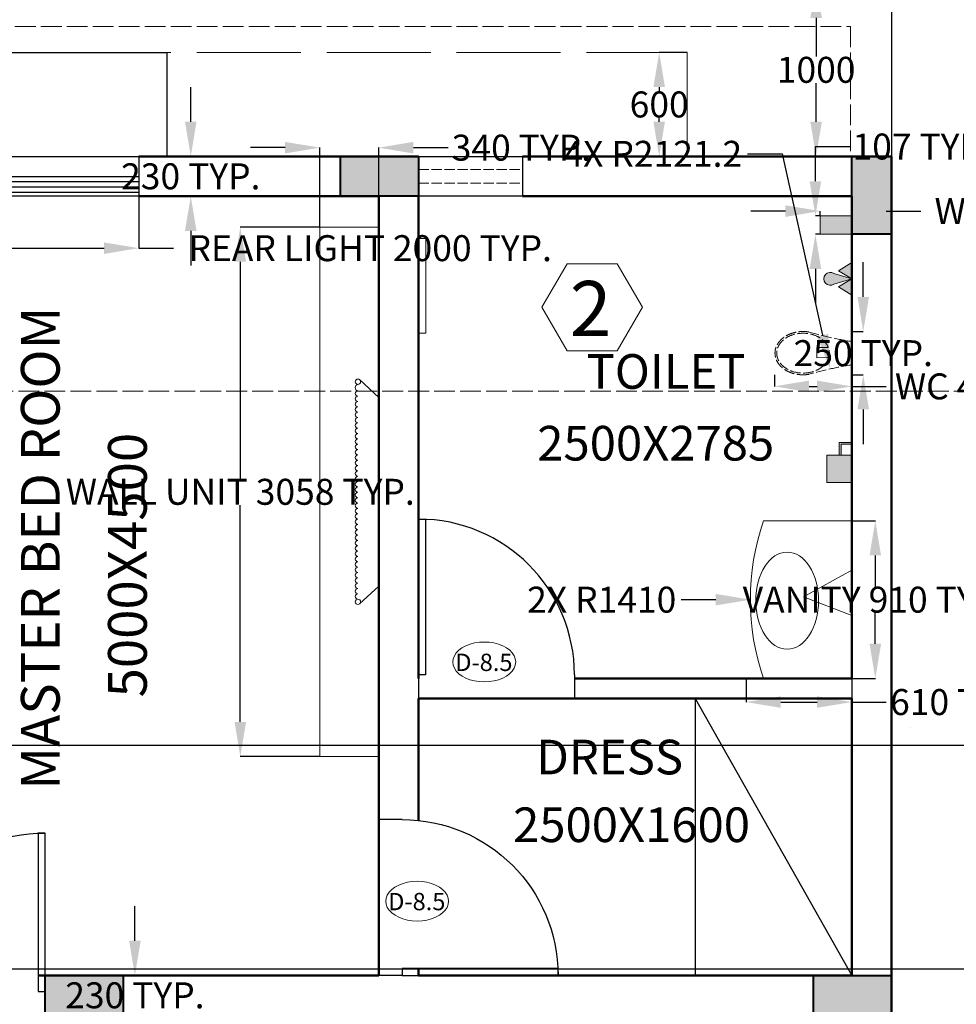
# Model space of a CAD drawing. Units: inches. Extents: x 22626 to 57351, y 2118 to 36234.
# Tile 8 of 10: x 44155 to 49561, y 23360 to 29046. Entities that reach past the tile are written whole.
import ezdxf

# ---------------------------------------------------------------- set-up
doc = ezdxf.new("R2010")
doc.units = ezdxf.units.IN
doc.header["$MEASUREMENT"] = 0
doc.linetypes.add('ACAD_ISO02W100', pattern=[15, 12, -3])
for name, color, linetype, lineweight in [('A-ANNO-DIMS', 130, 'Continuous', 18), ('A-ANNO-IDEN', 130, 'Continuous', 15), ('A-AREA-IDEN', 130, 'Continuous', 18), ('A-COLS', 7, 'Continuous', 40), ('A-COLS-PATT', 7, 'Continuous', 18), ('A-FLOR', 80, 'Continuous', 30), ('A-FLOR-CASE', 30, 'Continuous', 25), ('A-FLOR-FIXT', 30, 'Continuous', 18), ('A-FLOR-FIXT-HIDN', 30, 'ACAD_ISO02W100', 18), ('A-GLAZ-VENT', 152, 'Continuous', 25), ('A-GLAZ-VENT-HIDN', 152, 'ACAD_ISO02W100', 18), ('A-ROOF', 80, 'Continuous', 25), ('A-ROOF-OVHD', 80, 'ACAD_ISO02W100', 18), ('A-WALL', 80, 'Continuous', 50), ('DOORS', 32, 'Continuous', 25), ('FURNITURE', 30, 'Continuous', 18), ('WINDOWS', 212, 'Continuous', 25)]:
    doc.layers.add(name, color=color, linetype=linetype, lineweight=lineweight)
doc.layers.add('A-SECT', color=2, linetype='ACAD_ISO02W100', lineweight=18, true_color=0xf1eb1f)
doc.styles.get("Standard").update_dxf_attribs({"font": 'arial.ttf'})
doc.dimstyles.get("Standard").update_dxf_attribs({"dimtxt": 150, "dimasz": 200, "dimexe": 0.18, "dimexo": 0.0625, "dimgap": 0.09, "dimtad": 0, "dimtih": 1, "dimtoh": 1, "dimdec": 0, "dimzin": 0, "dimdsep": 46, "dimtxsty": 'Standard', "dimcen": 0.09, "dimadec": 0, "dimazin": 0, "dimtfac": 1, "dimtdec": 0, "dimtofl": 0, "dimtmove": 0, "dimatfit": 3, "dimfxl": 1, "dimtolj": 1, "dimtzin": 0, "dimarcsym": 0})

# ---------------------------------------------------------------- blocks, each defined once
blk = doc.blocks.new('*U7')
for p, q in [((0, 0), (-1e-16, -5.999999999999999)), ((40, -6e-16), (40, -6))]:
    blk.add_line(p, q)
blk.add_lwpolyline([(0, 0), (5.6e-15, 40), (1.750000000000007, 40), (1.749999999999998, -7e-16)], close=True)
blk.add_arc((0, 0), 40, 0, 90)
blk = doc.blocks.new('*D24')
at = {"layer": 'A-ANNO-DIMS', "color": 0, "lineweight": -2, "transparency": 16777216}
for p, q in [((48950.70212366983, 29256.86010836475), (48751.99162901918, 29256.86010836475)), ((48752.17162901917, 29056.86010836475), (48752.17162901917, 28833.536056523)), ((48752.17162901917, 28456.86010836475), (48752.17162901917, 28680.1841602065)), ((48950.70212366983, 28256.86010836474), (48751.99162901918, 28256.86010836474))]:
    blk.add_line(p, q, dxfattribs=at)
at = {"layer": 'A-ANNO-DIMS', "color": 0, "transparency": 16777216}
for points in [[(48718.83829568584, 29056.86010836475), (48785.50496235251, 29056.86010836475), (48752.17162901917, 29256.86010836475)], [(48718.83829568584, 28456.86010836475), (48785.50496235251, 28456.86010836475), (48752.17162901917, 28256.86010836474)]]:
    blk.add_solid(points, dxfattribs=at)
at = {"layer": 'Defpoints', "color": 0, "transparency": 16777216}
for p in [(48752.17162901917, 29256.86010836475), (48950.76462366983, 29256.86010836475), (48950.76462366983, 28256.86010836474)]:
    blk.add_point(p, dxfattribs=at)
at = {"layer": 'A-ANNO-DIMS', "color": 0, "transparency": 16777216, "insert": (48752.17162901917, 28756.86010836473), "char_height": 150, "attachment_point": 5}
blk.add_mtext('\\A1;1000', dxfattribs=at)
blk = doc.blocks.new('*D25')
at = {"layer": 'A-ANNO-DIMS', "color": 0, "lineweight": -2, "transparency": 16777216}
for p, q in [((48007.78103641213, 28856.86010836474), (47846.08778381056, 28856.86010836474)), ((47846.26778381056, 28656.86010836475), (47846.26778381056, 28633.536056523)), ((47846.26778381056, 28456.86010836475), (47846.26778381056, 28480.18416020649)), ((48007.78103641213, 28256.86010836474), (47846.08778381056, 28256.86010836474))]:
    blk.add_line(p, q, dxfattribs=at)
at = {"layer": 'A-ANNO-DIMS', "color": 0, "transparency": 16777216}
for points in [[(47812.93445047722, 28656.86010836475), (47879.6011171439, 28656.86010836475), (47846.26778381056, 28856.86010836474)], [(47812.93445047722, 28456.86010836475), (47879.6011171439, 28456.86010836475), (47846.26778381056, 28256.86010836474)]]:
    blk.add_solid(points, dxfattribs=at)
at = {"layer": 'Defpoints', "color": 0, "transparency": 16777216}
for p in [(47846.26778381056, 28856.86010836474), (48007.84353641212, 28856.86010836474), (48007.84353641212, 28256.86010836474)]:
    blk.add_point(p, dxfattribs=at)
at = {"layer": 'A-ANNO-DIMS', "color": 0, "transparency": 16777216, "insert": (47846.26778381056, 28556.86010836473), "char_height": 150, "attachment_point": 5}
blk.add_mtext('\\A1;600', dxfattribs=at)
blk = doc.blocks.new('BEDROOM-WALL-UNIT-LARGE')
for p, q in [((340.3900439586505, 2073.364799085331), (230.0040754163856, 2176.56373781851)), ((340.3900439586505, 2073.364799085331), (340.3900439586505, 984.3248137472802)), ((340.3900439586505, 984.3248137472802), (230.0040754163856, 881.1258750141023))]:
    blk.add_line(p, q)
blk.add_lwpolyline([(340.3900439586505, 3057.689448538677), (0.000138100287586, 3057.689448538677), (0.000138100287586, 0.0001642939350859), (340.3900439586505, 0.0001642939350859)], close=True)
for centre in [(220.3862887798459, 2164.500040820422), (220.3862887798459, 893.1895720121902)]:
    blk.add_circle(centre, 15.42837013581516)
for centre, radius, start, end in [((223.4783476155644, 2130.551241713074), 18.77677067903697, 99.47833690620159, 260.5216630937984), ((220.3862887798459, 2096.602442605719), 15.42837013581516, 90, 270), ((220.3862887798459, 2065.745702334091), 15.42837013581516, 90, 270), ((220.3862887798459, 2034.888962062462), 15.42837013581516, 90, 270), ((220.3862887798459, 2004.032221790833), 15.42837013581516, 90, 270), ((220.3862887798459, 1973.175481519203), 15.42837013581516, 90, 270), ((220.3862887798459, 1942.318741247574), 15.42837013581516, 90, 270), ((220.3862887798459, 1911.462000975945), 15.42837013581516, 90, 270), ((220.3862887798459, 1880.605260704317), 15.42837013581516, 90, 270), ((220.3862887798459, 1849.748520432688), 15.42837013581516, 90, 270), ((220.3862887798459, 1818.891780161058), 15.42837013581516, 90, 270), ((220.3862887798459, 1788.03503988943), 15.42837013581516, 90, 270), ((220.3862887798459, 1757.178299617801), 15.42837013581516, 90, 270), ((220.3862887798459, 1726.321559346172), 15.42837013581516, 90, 270), ((220.3862887798459, 1695.464819074543), 15.42837013581516, 90, 270), ((220.3862887798459, 1664.608078802914), 15.42837013581516, 90, 270), ((220.3862887798459, 1633.751338531285), 15.42837013581516, 90, 270), ((220.3862887798459, 1602.894598259656), 15.42837013581516, 90, 270), ((220.3862887798459, 1572.037857988027), 15.42837013581516, 90, 270), ((220.3862887798459, 1541.181117716398), 15.42837013581516, 90, 270), ((220.3862887798459, 1510.324377444769), 15.42837013581516, 90, 270), ((220.3862887798459, 1479.46763717314), 15.42837013581516, 90, 270), ((220.3862887798459, 1448.610896901511), 15.42837013581516, 90, 270), ((220.3862887798459, 1417.754156629882), 15.42837013581516, 90, 270), ((220.3862887798459, 1386.897416358253), 15.42837013581516, 90, 270), ((220.3862887798459, 1356.040676086624), 15.42837013581516, 90, 270), ((220.3862887798459, 1325.183935814995), 15.42837013581516, 90, 270), ((220.3862887798459, 1294.327195543366), 15.42837013581516, 90, 270), ((220.3862887798459, 1263.470455271737), 15.42837013581516, 90, 270), ((220.3862887798459, 1232.613715000108), 15.42837013581516, 90, 270), ((220.3862887798459, 1201.756974728479), 15.42837013581516, 90, 270), ((220.3862887798459, 1170.90023445685), 15.42837013581516, 90, 270), ((220.3862887798459, 1140.043494185221), 15.42837013581516, 90, 270), ((220.3862887798459, 1109.186753913593), 15.42837013581516, 90, 270), ((220.3862887798459, 1078.330013641964), 15.42837013581516, 90, 270), ((220.3862887798459, 1047.473273370335), 15.42837013581516, 90, 270), ((220.3862887798459, 1016.616533098706), 15.42837013581516, 90, 270), ((220.3862887798459, 985.759792827077), 15.42837013581516, 90, 270), ((220.3862887798459, 954.9030525554481), 15.42837013581516, 90, 270), ((220.3862887798459, 924.0463122838191), 15.42837013581516, 90, 270)]:
    blk.add_arc(centre, radius, start, end)
blk = doc.blocks.new('WC')
at = {"ltscale": 5}
for p, q in [((307.4540408789253, 157.9229967620813), (242.2174300020561, 157.9229967620813)), ((242.2174300020561, 157.9229967620813), (242.2174300020561, 97.87988847275483)), ((307.4540408789253, 157.9229967620813), (307.4540408789253, 157.9229967620813)), ((242.2174300020561, 97.87988847275483), (310.0842174796853, 99.70460823710528))]:
    blk.add_line(p, q, dxfattribs=at)
for centre, start, end in [((780.732508801062, 2286.288249576111), 254.000576969056, 260.8285458946419), ((780.732508801062, -2036.267674000785), 99.17145410535805, 105.999423030944)]:
    blk.add_arc(centre, 2121.236142909723, start, end, dxfattribs=at)
blk.add_ellipse((161.9027973060947, 125.0102877876634), major_axis=(151.9040759523413, 0), ratio=0.7571275708385353, start_param=-1.570796326794896, end_param=4.712388980384689, dxfattribs=at)
for points, knots in [([(196.0611207178517, 247.2193096078299), (189.9898489161132, 248.2266596507652), (183.8456655129121, 248.9650412442752), (168.6182293347155, 250.1102459839712), (159.4964975931143, 250.2034131541222), (141.3581357193834, 249.212698022955), (132.3417047420516, 248.1288311957833), (114.6613914742556, 244.8098406800164), (105.9976853845146, 242.5747636017513), (89.26201623554518, 237.0062334978611), (81.19018288652298, 233.6728365616509), (65.86452451616788, 225.9859897466813), (58.61077128878969, 221.6325587335632), (45.13156838521536, 212.0080719868456), (38.90616664764093, 206.7369257869286), (27.67640637096338, 195.4043234284545), (22.67220516936504, 189.3426231032536), (14.05759261523781, 176.5860631599644), (10.44766267286468, 169.8909471035294), (4.765577569938614, 156.0629077761186), (2.69424158098991, 148.9301527436837), (0.1846293913040426, 134.463597005164), (-0.2530317139462568, 127.1307025187488), (0.5271766823570943, 112.5265070110981), (1.744832412616233, 105.2563518462193), (5.77749157987273, 91.03263116568269), (8.591685077881264, 84.07962673572185), (15.69573821845551, 70.70922901844096), (19.98490811580268, 64.29173781119243), (29.87879523489392, 52.16900764399179), (35.483208879421, 46.46348057011346), (47.82439502190391, 35.90657261581146), (54.56108629030495, 31.05501885116246), (68.96556532807881, 22.32099587028279), (76.63330319123634, 18.43849746629348), (92.68186228567357, 11.73355477496807), (101.0625846676266, 8.91115468616772), (118.3043576900527, 4.392898517646244), (127.1652540279829, 2.697098106120392), (144.6597339432555, 0.5298149587142689), (153.2812269904534, -0.000476238605188), (161.9027973060947, -0.000476238605188)], [1.35503494441986, 1.35503494441986, 1.35503494441986, 1.35503494441986, 1.471789532681877, 1.471789532681877, 1.642812487519809, 1.642812487519809, 1.813835442357741, 1.813835442357741, 1.984858397195673, 1.984858397195673, 2.155881352033606, 2.155881352033606, 2.326904306871538, 2.326904306871538, 2.49792726170947, 2.49792726170947, 2.668950216547402, 2.668950216547402, 2.839973171385334, 2.839973171385334, 3.010996126223266, 3.010996126223266, 3.182019081061198, 3.182019081061198, 3.35304203589913, 3.35304203589913, 3.524064990737062, 3.524064990737062, 3.695087945574994, 3.695087945574994, 3.866110900412926, 3.866110900412926, 4.037133855250859, 4.037133855250859, 4.208156810088791, 4.208156810088791, 4.379179764926723, 4.379179764926723, 4.550202719764655, 4.550202719764655, 4.712388980384689, 4.712388980384689, 4.712388980384689, 4.712388980384689]), ([(161.9027973060947, -0.000476238605188), (167.8851873344465, -0.000476238605188), (173.8675648995122, 0.254611844480678), (185.2699231324077, 1.230286525809788), (190.6953945214336, 1.911114408936555), (196.0639028232108, 2.802063691000512)], [-1.570796326794896, -1.570796326794896, -1.570796326794896, -1.570796326794896, -1.458257493061962, -1.458257493061962, -1.355016516099114, -1.355016516099114, -1.355016516099114, -1.355016516099114])]:
    blk.add_open_spline(points, degree=3, knots=knots, dxfattribs=at)
blk = doc.blocks.new('VANITY-BASIN')
for p, q in [((584.7220439586453, 910.0402479339828), (75.43762569876708, 910.0402479339828)), ((305.8230790732414, 471.9850997598696), (584.7220439586453, 624.7406586797733)), ((305.8230790732414, 471.9850997598696), (584.7220439586453, 362.8739423048537))]:
    blk.add_line(p, q)
blk.add_arc((1409.991080111897, 455.0201781493488), 1409.991555504085, 161.1730336158717, 198.8269663841282)
blk.add_ellipse((212.5566461408889, 449.1359101998277), major_axis=(0, -280.3059750137254), ratio=0.6469075979310198)
blk = doc.blocks.new('WIN-FIXED-2000-REAR')
for p, q in [((4.39586510765e-05, 114.2630103577103), (2000.000043958651, 114.2630103577103)), ((4.39586510765e-05, 84.26301035771031), (2000.000043958651, 84.26301035771031)), ((4.39586510765e-05, 54.2630103577103), (2000.000043958651, 54.2630103577103)), ((4.39586510765e-05, 24.2630103577103), (2000.000043958651, 24.2630103577103))]:
    blk.add_line(p, q)
blk.add_lwpolyline([(4.39586510765e-05, 230.0001083647294), (2000.000043958651, 230.0001083647294), (2000.000043958651, 0.0001083647330233), (4.39586438006e-05, 0.0001083647330233), (4.39586510765e-05, 230.0001083647294)])
blk = doc.blocks.new('COL-RECTANGULAR')
h = blk.add_hatch(color=256)
h.dxf.hatch_style = 1
h.paths.add_polyline_path([(4.39586474386e-05, 0.0001083647293854), (450.0000439586474, 0.0001083647293854), (450.0000439586474, 230.0001083647294), (4.39586474386e-05, 230.0001083647294)])
blk.add_lwpolyline([(4.39586474386e-05, 0.0001083647293854), (4.39586474386e-05, 230.0001083647294), (450.0000439586474, 230.0001083647294), (450.0000439586474, 0.0001083647293854)], close=True)
blk = doc.blocks.new('BATH-SUPPLY-FITTING')
h = blk.add_hatch(color=256)
h.dxf.hatch_style = 1
h.paths.add_polyline_path([(161.0140439586466, 189.3806798614205), (84.84003036547074, 140.983449503361), (161.0140439586466, 94.69046873241678)])
h = blk.add_hatch(color=256)
h.dxf.hatch_style = 1
h.paths.add_polyline_path([(161.0140439586466, 94.69046873241678), (58.24591656582924, 125.2086534748123, 1.90856376211952), (58.24591656582924, 64.17228399002124)])
h = blk.add_hatch(color=256)
h.dxf.hatch_style = 1
h.paths.add_polyline_path([(161.0140439586466, 94.69046873241678), (84.84003036547074, 48.39748796147251), (161.0140439586466, 0.000257603413047)])
for p, q in [((161.0140439586466, 189.3806798614205), (84.84003036547074, 140.983449503361)), ((161.0140439586466, 94.69046873241678), (58.24591656582924, 125.2086534748123)), ((84.84003036547074, 140.983449503361), (161.0140439586466, 94.69046873241678)), ((161.0140439586466, 94.69046873241678), (58.24591656582924, 64.17228399002124)), ((84.84003036547074, 48.39748796147251), (161.0140439586466, 94.69046873241678)), ((161.0140439586466, 0.000257603413047), (84.84003036547074, 48.39748796147251))]:
    blk.add_line(p, q)
blk.add_arc((37.11803136635718, 94.69046873241678), 37.11801628553248, 55.30495923588778, 304.6950407641123)
blk = doc.blocks.new('BATH-WALL-ACCESSORY')
h = blk.add_hatch(color=256)
h.dxf.hatch_style = 1
h.paths.add_polyline_path([(142.8430439586445, 231.1050653827879), (71.42162994010141, 231.1050653827879), (71.42162994010141, 158.5160872540764), (81.4216299401014, 158.5160872540764), (81.42162994010869, 221.1050653827879), (142.8430439586445, 221.1050653827879)])
h = blk.add_hatch(color=256)
h.dxf.hatch_style = 1
h.paths.add_polyline_path([(142.8430439586445, 158.5160872540764), (0.0002159215582651, 158.5160872540764), (0.0002159215582651, -1.22242890939e-05), (142.8430439586445, -1.22242854559e-05)])
for p, q in [((71.42162994010141, 158.5160872540764), (71.42162994010141, 231.1050653827879)), ((71.42162994010141, 231.1050653827879), (142.8430439586445, 231.1050653827879)), ((81.42162994010869, 221.1050653827879), (142.8430439586445, 221.1050653827879)), ((81.4216299401014, 158.5160872540764), (81.42162994010869, 221.1050653827879)), ((142.8430439586445, 158.5160872540764), (0.0002159215582651, 158.5160872540764)), ((0.0002159215582651, 158.5160872540764), (0.0002159215582651, -1.22242890939e-05)), ((142.8430439586445, 158.5160872540764), (142.8430439586445, 158.5160872540764)), ((0.0002159215582651, -1.22242890939e-05), (142.8430439586445, -1.22242854559e-05))]:
    blk.add_line(p, q)
blk = doc.blocks.new('BATH-WALL-BOX')
h = blk.add_hatch(color=256)
h.dxf.hatch_style = 1
h.paths.add_polyline_path([(182.0210439586444, 106.8341357510071), (0.000183795193152, 106.8341357510071), (0.000183795193152, 0.0001083647293854), (182.0210439586444, 0.0001083647293854)])
for p, q in [((0.000183795193152, 0.0001083647293854), (0.000183795193152, 106.8341357510071)), ((0.000183795193152, 106.8341357510071), (182.0210439586444, 106.8341357510071)), ((182.0210439586444, 0.0001083647293854), (0.000183795193152, 0.0001083647293854))]:
    blk.add_line(p, q)
blk = doc.blocks.new('WINDOW-HOOD')
for p, q in [((-0.0002120264252881, 0.0001083647293854), (-0.0002120264252881, 600.0001083647293)), ((-0.0002120264252881, 600.0001083647293), (2314.590014351226, 600.0001083647293)), ((2314.590014351226, 600.0001083647293), (2314.590014351226, 0.0001083647330233))]:
    blk.add_line(p, q)
blk = doc.blocks.new('*D56')
at = {"layer": 'A-ANNO-DIMS', "color": 0, "lineweight": -2, "transparency": 16777216}
for p, q in [((44302.42904395863, 23296.79760836473), (44302.42904395863, 23229.18010836473)), ((44752.42904395862, 23296.79760836473), (44752.42904395862, 23229.18010836473)), ((44502.42904395863, 23229.36010836473), (44552.42904395862, 23229.36010836473)), ((44752.42904395862, 23229.36010836473), (44952.42904395862, 23229.36010836473))]:
    blk.add_line(p, q, dxfattribs=at)
at = {"layer": 'A-ANNO-DIMS', "color": 0, "transparency": 16777216}
for points in [[(44502.42904395863, 23262.69344169806), (44502.42904395863, 23196.0267750314), (44302.42904395863, 23229.36010836473)], [(44552.42904395862, 23262.69344169806), (44552.42904395862, 23196.0267750314), (44752.42904395862, 23229.36010836473)]]:
    blk.add_solid(points, dxfattribs=at)
at = {"layer": 'Defpoints', "color": 0, "transparency": 16777216}
for p in [(44302.42904395863, 23296.86010836473), (44752.42904395862, 23296.86010836473), (44752.42904395862, 23229.36010836473)]:
    blk.add_point(p, dxfattribs=at)
at = {"layer": 'A-ANNO-DIMS', "color": 0, "transparency": 16777216, "insert": (45858.14660193952, 23229.36010836473), "char_height": 150, "attachment_point": 5}
blk.add_mtext('\\A1;COLUMN 450 TYP.', dxfattribs=at)
blk = doc.blocks.new('*D57')
at = {"layer": 'A-ANNO-DIMS', "color": 0, "lineweight": -2, "transparency": 16777216}
for p, q in [((44819.92904395865, 23726.86010836474), (44819.92904395865, 23926.86010836474)), ((44752.49154395863, 23526.86010836474), (44820.10904395865, 23526.86010836474)), ((44752.49154395863, 23296.86010836474), (44820.10904395865, 23296.86010836474)), ((44819.92904395865, 23096.86010836474), (44819.92904395865, 22896.86010836474))]:
    blk.add_line(p, q, dxfattribs=at)
at = {"layer": 'A-ANNO-DIMS', "color": 0, "transparency": 16777216}
for points in [[(44786.59571062531, 23726.86010836474), (44853.26237729199, 23726.86010836474), (44819.92904395865, 23526.86010836474)], [(44786.59571062531, 23096.86010836474), (44853.26237729199, 23096.86010836474), (44819.92904395865, 23296.86010836474)]]:
    blk.add_solid(points, dxfattribs=at)
at = {"layer": 'Defpoints', "color": 0, "transparency": 16777216}
for p in [(44752.42904395864, 23526.86010836474), (44819.92904395865, 23526.86010836474), (44752.42904395864, 23296.86010836474)]:
    blk.add_point(p, dxfattribs=at)
at = {"layer": 'A-ANNO-DIMS', "color": 0, "transparency": 16777216, "insert": (44819.92904395865, 23411.86010836472), "char_height": 150, "attachment_point": 5}
blk.add_mtext('\\A1;230 TYP.', dxfattribs=at)
blk = doc.blocks.new('*D62')
at = {"layer": 'A-ANNO-DIMS', "color": 0, "lineweight": -2, "transparency": 16777216}
for p, q in [((48511.89638763924, 26995.3910237614), (48511.89638763924, 26928.44362531275)), ((48957.42904396353, 26995.3910237614), (48957.42904396353, 26928.44362531275)), ((48711.89638763923, 26928.62362531275), (48757.42904396354, 26928.62362531275)), ((48957.42904396353, 26928.62362531275), (49157.42904396354, 26928.62362531275))]:
    blk.add_line(p, q, dxfattribs=at)
at = {"layer": 'A-ANNO-DIMS', "color": 0, "transparency": 16777216}
for points in [[(48711.89638763923, 26961.95695864608), (48711.89638763923, 26895.29029197942), (48511.89638763924, 26928.62362531275)], [(48757.42904396354, 26961.95695864608), (48757.42904396354, 26895.29029197942), (48957.42904396353, 26928.62362531275)]]:
    blk.add_solid(points, dxfattribs=at)
at = {"layer": 'Defpoints', "color": 0, "transparency": 16777216}
for p in [(48511.89638763924, 26995.4535237614), (48957.42904396353, 26995.4535237614), (48957.42904396353, 26928.62362531275)]:
    blk.add_point(p, dxfattribs=at)
at = {"layer": 'A-ANNO-DIMS', "color": 0, "transparency": 16777216, "insert": (49787.60089935235, 26928.62362531275), "char_height": 150, "attachment_point": 5}
blk.add_mtext('\\A1;WC 446 TYP.', dxfattribs=at)
blk = doc.blocks.new('*D63')
at = {"layer": 'A-ANNO-DIMS', "color": 0, "lineweight": -2, "transparency": 16777216}
for p, q in [((49024.25894241221, 27445.65741315414), (49024.25894241221, 27645.65741315414)), ((48957.49154396355, 27245.65741315414), (49024.43894241221, 27245.65741315414)), ((48957.49154396355, 26995.45352376141), (49024.43894241221, 26995.45352376141)), ((49024.25894241221, 26795.45352376141), (49024.25894241221, 26595.45352376141))]:
    blk.add_line(p, q, dxfattribs=at)
at = {"layer": 'A-ANNO-DIMS', "color": 0, "transparency": 16777216}
for points in [[(48990.92560907887, 27445.65741315414), (49057.59227574555, 27445.65741315414), (49024.25894241221, 27245.65741315414)], [(48990.92560907887, 26795.45352376141), (49057.59227574555, 26795.45352376141), (49024.25894241221, 26995.45352376141)]]:
    blk.add_solid(points, dxfattribs=at)
at = {"layer": 'Defpoints', "color": 0, "transparency": 16777216}
for p in [(48957.42904396355, 27245.65741315414), (49024.25894241221, 27245.65741315414), (48957.42904396355, 26995.45352376141)]:
    blk.add_point(p, dxfattribs=at)
at = {"layer": 'A-ANNO-DIMS', "color": 0, "transparency": 16777216, "insert": (49024.25894241221, 27120.55546845776), "char_height": 150, "attachment_point": 5}
blk.add_mtext('\\A1;250 TYP.', dxfattribs=at)
blk = doc.blocks.new('*D64')
at = {"layer": 'A-ANNO-DIMS', "color": 0, "lineweight": -2, "transparency": 16777216}
for p, q in [((48957.49154395866, 26151.900247934), (49094.1150648939, 26151.900247934)), ((49093.9350648939, 25951.900247934), (49093.9350648939, 25773.55612630816)), ((49093.9350648939, 25441.86010836582), (49093.9350648939, 25620.20422999166)), ((48957.49154395866, 25241.86010836582), (49094.1150648939, 25241.86010836582))]:
    blk.add_line(p, q, dxfattribs=at)
at = {"layer": 'A-ANNO-DIMS', "color": 0, "transparency": 16777216}
for points in [[(49060.60173156056, 25951.900247934), (49127.26839822723, 25951.900247934), (49093.9350648939, 26151.900247934)], [(49060.60173156056, 25441.86010836582), (49127.26839822723, 25441.86010836582), (49093.9350648939, 25241.86010836582)]]:
    blk.add_solid(points, dxfattribs=at)
at = {"layer": 'Defpoints', "color": 0, "transparency": 16777216}
for p in [(48957.42904395866, 26151.900247934), (49093.9350648939, 26151.900247934), (48957.42904395866, 25241.86010836582)]:
    blk.add_point(p, dxfattribs=at)
at = {"layer": 'A-ANNO-DIMS', "color": 0, "transparency": 16777216, "insert": (49093.9350648939, 25696.88017814989), "char_height": 150, "attachment_point": 5}
blk.add_mtext('\\A1;VANITY 910 TYP.', dxfattribs=at)
blk = doc.blocks.new('*D65')
at = {"layer": 'A-ANNO-DIMS', "color": 0, "lineweight": -2, "transparency": 16777216}
for p, q in [((48347.56049091095, 25241.79760836581), (48347.56049091095, 25105.17408743058)), ((48957.42904395865, 25241.79760836581), (48957.42904395865, 25105.17408743058)), ((48547.56049091095, 25105.35408743058), (48757.42904395864, 25105.35408743058)), ((48957.42904395865, 25105.35408743058), (49157.42904395864, 25105.35408743058))]:
    blk.add_line(p, q, dxfattribs=at)
at = {"layer": 'A-ANNO-DIMS', "color": 0, "transparency": 16777216}
for points in [[(48547.56049091095, 25138.68742076391), (48547.56049091095, 25072.02075409725), (48347.56049091095, 25105.35408743058)], [(48757.42904395864, 25138.68742076391), (48757.42904395864, 25072.02075409725), (48957.42904395865, 25105.35408743058)]]:
    blk.add_solid(points, dxfattribs=at)
at = {"layer": 'Defpoints', "color": 0, "transparency": 16777216}
for p in [(48347.56049091095, 25241.86010836581), (48957.42904395865, 25241.86010836581), (48957.42904395865, 25105.35408743058)]:
    blk.add_point(p, dxfattribs=at)
at = {"layer": 'A-ANNO-DIMS', "color": 0, "transparency": 16777216, "insert": (49581.27415992044, 25105.35408743058), "char_height": 150, "attachment_point": 5}
blk.add_mtext('\\A1;610 TYP.', dxfattribs=at)
blk = doc.blocks.new('*D70')
at = {"layer": 'A-ANNO-DIMS', "color": 0, "lineweight": -2, "transparency": 16777216}
for p, q in [((48575.4081837952, 27940.99726477552), (48375.4081837952, 27940.99726477552)), ((48775.4081837952, 27913.75663575101), (48775.4081837952, 27941.17726477553)), ((48957.42904395865, 27913.75663575101), (48957.42904395865, 27941.17726477553)), ((49157.42904395864, 27940.99726477552), (49357.42904395865, 27940.99726477552))]:
    blk.add_line(p, q, dxfattribs=at)
at = {"layer": 'A-ANNO-DIMS', "color": 0, "transparency": 16777216}
for points in [[(48575.4081837952, 27974.33059810886), (48575.4081837952, 27907.66393144219), (48775.4081837952, 27940.99726477552)], [(49157.42904395864, 27974.33059810886), (49157.42904395864, 27907.66393144219), (48957.42904395865, 27940.99726477552)]]:
    blk.add_solid(points, dxfattribs=at)
at = {"layer": 'Defpoints', "color": 0, "transparency": 16777216}
for p in [(48957.42904395865, 27940.99726477552), (48775.4081837952, 27913.69413575101), (48957.42904395865, 27913.69413575101)]:
    blk.add_point(p, dxfattribs=at)
at = {"layer": 'A-ANNO-DIMS', "color": 0, "transparency": 16777216, "insert": (50348.73664286724, 27940.99726477552), "char_height": 150, "attachment_point": 5}
blk.add_mtext('\\A1;WALL BOX 182 TYP.', dxfattribs=at)
blk = doc.blocks.new('*D71')
at = {"layer": 'A-ANNO-DIMS', "color": 0, "lineweight": -2, "transparency": 16777216}
for p, q in [((48748.1050547707, 28113.69413575102), (48748.1050547707, 28313.69413575102)), ((48748.1050547707, 28313.69413575102), (48948.10505477069, 28313.69413575102)), ((48775.34568379521, 27913.69413575102), (48747.9250547707, 27913.69413575102)), ((48775.34568379521, 27806.86010836475), (48747.9250547707, 27806.86010836475)), ((48748.1050547707, 27606.86010836475), (48748.1050547707, 27406.86010836475))]:
    blk.add_line(p, q, dxfattribs=at)
at = {"layer": 'A-ANNO-DIMS', "color": 0, "transparency": 16777216}
for points in [[(48714.77172143736, 28113.69413575102), (48781.43838810403, 28113.69413575102), (48748.1050547707, 27913.69413575102)], [(48714.77172143736, 27606.86010836475), (48781.43838810403, 27606.86010836475), (48748.1050547707, 27806.86010836475)]]:
    blk.add_solid(points, dxfattribs=at)
at = {"layer": 'Defpoints', "color": 0, "transparency": 16777216}
for p in [(48748.1050547707, 27913.69413575102), (48775.40818379522, 27913.69413575102), (48775.40818379522, 27806.86010836475)]:
    blk.add_point(p, dxfattribs=at)
at = {"layer": 'A-ANNO-DIMS', "color": 0, "transparency": 16777216, "insert": (49364.4808665033, 28313.694135751), "char_height": 150, "attachment_point": 5}
blk.add_mtext('\\A1;107 TYP.', dxfattribs=at)
blk = doc.blocks.new('*D78')
at = {"layer": 'A-ANNO-DIMS', "color": 0, "lineweight": -2, "transparency": 16777216}
for p, q in [((45886.97663810028, 27848.6944485387), (45428.20574546359, 27848.6944485387)), ((45428.38574546359, 27648.6944485387), (45428.38574546359, 26396.57691419259)), ((45428.38574546359, 24991.00516429395), (45428.38574546359, 26243.12269864006)), ((45886.97663810028, 24791.00516429395), (45428.20574546359, 24791.00516429395))]:
    blk.add_line(p, q, dxfattribs=at)
at = {"layer": 'A-ANNO-DIMS', "color": 0, "transparency": 16777216}
for points in [[(45395.05241213025, 27648.6944485387), (45461.71907879693, 27648.6944485387), (45428.38574546359, 27848.6944485387)], [(45395.05241213025, 24991.00516429395), (45461.71907879693, 24991.00516429395), (45428.38574546359, 24791.00516429395)]]:
    blk.add_solid(points, dxfattribs=at)
at = {"layer": 'Defpoints', "color": 0, "transparency": 16777216}
for p in [(45428.38574546359, 27848.6944485387), (45887.03913810029, 27848.6944485387), (45887.03913810029, 24791.00516429395)]:
    blk.add_point(p, dxfattribs=at)
at = {"layer": 'A-ANNO-DIMS', "color": 0, "transparency": 16777216, "insert": (45428.38574546359, 26319.8498064163), "char_height": 150, "attachment_point": 5}
blk.add_mtext('\\A1;WALL UNIT 3058 TYP.', dxfattribs=at)
blk = doc.blocks.new('*D79')
at = {"layer": 'A-ANNO-DIMS', "color": 0, "lineweight": -2, "transparency": 16777216}
for p, q in [((45687.03913810027, 28307.34784117539), (45487.03913810028, 28307.34784117539)), ((45887.03913810028, 27848.75694853868), (45887.03913810028, 28307.52784117539)), ((46227.42904395864, 27848.75694853868), (46227.42904395864, 28307.52784117539)), ((46427.42904395864, 28307.34784117539), (46627.42904395864, 28307.34784117539))]:
    blk.add_line(p, q, dxfattribs=at)
at = {"layer": 'A-ANNO-DIMS', "color": 0, "transparency": 16777216}
for points in [[(45687.03913810027, 28340.68117450872), (45687.03913810027, 28274.01450784206), (45887.03913810028, 28307.34784117539)], [(46427.42904395864, 28340.68117450872), (46427.42904395864, 28274.01450784206), (46227.42904395864, 28307.34784117539)]]:
    blk.add_solid(points, dxfattribs=at)
at = {"layer": 'Defpoints', "color": 0, "transparency": 16777216}
for p in [(46227.42904395864, 28307.34784117539), (45887.03913810028, 27848.69444853868), (46227.42904395864, 27848.69444853868)]:
    blk.add_point(p, dxfattribs=at)
at = {"layer": 'A-ANNO-DIMS', "color": 0, "transparency": 16777216, "insert": (47050.81372335837, 28307.34784117539), "char_height": 150, "attachment_point": 5}
blk.add_mtext('\\A1;340 TYP.', dxfattribs=at)
blk = doc.blocks.new('*D82')
at = {"layer": 'A-ANNO-DIMS', "color": 0, "lineweight": -2, "transparency": 16777216}
for p, q in [((42842.42904395863, 28026.79760836474), (42842.42904395863, 27726.68010836474)), ((44842.42904395864, 28026.79760836474), (44842.42904395864, 27726.68010836474)), ((43042.42904395863, 27726.86010836474), (44642.42904395864, 27726.86010836474)), ((44842.42904395864, 27726.86010836474), (45042.42904395864, 27726.86010836474))]:
    blk.add_line(p, q, dxfattribs=at)
at = {"layer": 'A-ANNO-DIMS', "color": 0, "transparency": 16777216}
for points in [[(43042.42904395863, 27760.19344169807), (43042.42904395863, 27693.52677503141), (42842.42904395863, 27726.86010836474)], [(44642.42904395864, 27760.19344169807), (44642.42904395864, 27693.52677503141), (44842.42904395864, 27726.86010836474)]]:
    blk.add_solid(points, dxfattribs=at)
at = {"layer": 'Defpoints', "color": 0, "transparency": 16777216}
for p in [(42842.42904395863, 28026.86010836474), (44842.42904395864, 28026.86010836474), (44842.42904395864, 27726.86010836474)]:
    blk.add_point(p, dxfattribs=at)
at = {"layer": 'A-ANNO-DIMS', "color": 0, "transparency": 16777216, "insert": (46178.10908488633, 27726.86010836474), "char_height": 150, "attachment_point": 5}
blk.add_mtext('\\A1;REAR LIGHT 2000 TYP.', dxfattribs=at)
blk = doc.blocks.new('*D83')
at = {"layer": 'A-ANNO-DIMS', "color": 0, "lineweight": -2, "transparency": 16777216}
for p, q in [((45142.42904395866, 28456.86010836475), (45142.42904395866, 28656.86010836475)), ((44842.49154395866, 28256.86010836474), (45142.60904395866, 28256.86010836474)), ((44842.49154395866, 28026.86010836475), (45142.60904395866, 28026.86010836475)), ((45142.42904395866, 27826.86010836475), (45142.42904395866, 27626.86010836475))]:
    blk.add_line(p, q, dxfattribs=at)
at = {"layer": 'A-ANNO-DIMS', "color": 0, "transparency": 16777216}
for points in [[(45109.09571062533, 28456.86010836475), (45175.762377292, 28456.86010836475), (45142.42904395866, 28256.86010836474)], [(45109.09571062533, 27826.86010836475), (45175.762377292, 27826.86010836475), (45142.42904395866, 28026.86010836475)]]:
    blk.add_solid(points, dxfattribs=at)
at = {"layer": 'Defpoints', "color": 0, "transparency": 16777216}
for p in [(44842.42904395865, 28256.86010836474), (45142.42904395866, 28256.86010836474), (44842.42904395865, 28026.86010836475)]:
    blk.add_point(p, dxfattribs=at)
at = {"layer": 'A-ANNO-DIMS', "color": 0, "transparency": 16777216, "insert": (45142.42904395866, 28141.86010836473), "char_height": 150, "attachment_point": 5}
blk.add_mtext('\\A1;230 TYP.', dxfattribs=at)
blk = doc.blocks.new('*D99')
at = {"layer": 'A-ANNO-DIMS', "color": 0, "lineweight": -2, "transparency": 16777216}
for p, q in [((41184.594559, 30456.86010800002), (57038.79342100006, 30456.86010800002)), ((57038.61342100005, 30256.86010800002), (57038.61342100005, 18933.58721577627)), ((57038.61342100006, 7456.860108000005), (57038.61342100005, 18780.13300022374)), ((43702.49154400001, 7256.860108000004), (57038.79342100006, 7256.860108000005))]:
    blk.add_line(p, q, dxfattribs=at)
at = {"layer": 'A-ANNO-DIMS', "color": 0, "transparency": 16777216}
for points in [[(57005.28008766672, 30256.86010800002), (57071.94675433339, 30256.86010800002), (57038.61342100005, 30456.86010800002)], [(57005.28008766673, 7456.860108000005), (57071.9467543334, 7456.860108000005), (57038.61342100006, 7256.860108000005)]]:
    blk.add_solid(points, dxfattribs=at)
at = {"layer": 'Defpoints', "color": 0, "transparency": 16777216}
for p in [(41184.53205900001, 30456.86010800002), (57038.61342100005, 30456.86010800002), (43702.42904400001, 7256.860108000004)]:
    blk.add_point(p, dxfattribs=at)
at = {"layer": 'A-ANNO-DIMS', "color": 0, "transparency": 16777216, "insert": (57038.61342100005, 18856.86010799999), "char_height": 150, "attachment_point": 5}
blk.add_mtext('\\A1;23200', dxfattribs=at)
blk = doc.blocks.new('*D109')
at = {"layer": 'A-ANNO-DIMS', "color": 0, "lineweight": -2, "transparency": 16777216}
for p, q in [((38641.09672300002, 24856.10781600001), (57038.79342100006, 24856.10781600002)), ((57038.61342100005, 24656.10781600002), (57038.61342100005, 24287.47888015827)), ((57038.61342100005, 23765.49804800001), (57038.61342100005, 24134.12698384176)), ((38641.09672300002, 23565.49804800001), (57038.79342100006, 23565.49804800001))]:
    blk.add_line(p, q, dxfattribs=at)
at = {"layer": 'A-ANNO-DIMS', "color": 0, "transparency": 16777216}
for points in [[(57005.28008766672, 24656.10781600002), (57071.94675433339, 24656.10781600002), (57038.61342100005, 24856.10781600002)], [(57005.28008766672, 23765.49804800001), (57071.94675433339, 23765.49804800001), (57038.61342100005, 23565.49804800001)]]:
    blk.add_solid(points, dxfattribs=at)
at = {"layer": 'Defpoints', "color": 0, "transparency": 16777216}
for p in [(38641.03422300002, 24856.10781600001), (57038.61342100005, 24856.10781600002), (38641.03422300002, 23565.49804800001)]:
    blk.add_point(p, dxfattribs=at)
at = {"layer": 'A-ANNO-DIMS', "color": 0, "transparency": 16777216, "insert": (57038.61342100005, 24210.802932), "char_height": 150, "attachment_point": 5}
blk.add_mtext('\\A1;1290.6', dxfattribs=at)
blk = doc.blocks.new('*D114')
at = {"layer": 'A-ANNO-DIMS', "color": 0, "lineweight": -2, "transparency": 16777216}
for p, q in [((48355.99959704684, 28271.61414499024), (48555.99959704685, 28271.61414499024)), ((48555.99959704685, 28271.61414499024), (48789.74499842099, 27224.64814182229)), ((49295.44150900001, 24959.186326), (49295.621509, 24959.186326)), ((49295.53150900001, 24959.096326), (49295.53150900001, 24959.276326))]:
    blk.add_line(p, q, dxfattribs=at)
at = {"layer": 'A-ANNO-DIMS', "color": 0, "transparency": 16777216}
blk.add_solid([(48822.27740322471, 27231.9113194188), (48757.21259361728, 27217.38496422579), (48833.32406400001, 27029.453713)], dxfattribs=at)
at = {"layer": 'Defpoints', "color": 0, "transparency": 16777216}
for p in [(48833.32406400001, 27029.453713), (49295.53150900002, 24959.186326)]:
    blk.add_point(p, dxfattribs=at)
at = {"layer": 'A-ANNO-DIMS', "color": 0, "transparency": 16777216, "insert": (47809.37139786539, 28271.61414499024), "char_height": 150, "attachment_point": 5}
blk.add_mtext('\\A1;4X R2121.2', dxfattribs=at)
blk = doc.blocks.new('*D115')
at = {"layer": 'A-ANNO-DIMS', "color": 0, "lineweight": -2, "transparency": 16777216}
for p, q in [((47972.70652499999, 25696.88), (48172.706525, 25696.88)), ((49782.60808, 25696.880178), (49782.78807999999, 25696.880178)), ((49782.69808, 25696.790178), (49782.69808, 25696.970178))]:
    blk.add_line(p, q, dxfattribs=at)
at = {"layer": 'A-ANNO-DIMS', "color": 0, "transparency": 16777216}
blk.add_solid([(48172.706525, 25730.21333333334), (48172.706525, 25663.54666666667), (48372.70652499999, 25696.88)], dxfattribs=at)
at = {"layer": 'Defpoints', "color": 0, "transparency": 16777216}
for p in [(48372.70652499999, 25696.88), (49782.69808, 25696.880178)]:
    blk.add_point(p, dxfattribs=at)
at = {"layer": 'A-ANNO-DIMS', "color": 0, "transparency": 16777216, "insert": (47514.68678420873, 25696.88), "char_height": 150, "attachment_point": 5}
blk.add_mtext('\\A1;2X R1410', dxfattribs=at)

msp = doc.modelspace()

# ---------------------------------------------------------------- hatches: boundary and pattern name
at = {"layer": 'A-COLS-PATT'}
h = msp.add_hatch(color=256, dxfattribs=at)
h.dxf.hatch_style = 1
h.paths.add_polyline_path([(49187.42904395864, 28256.86010836473), (48957.42904395865, 28256.86010836473), (48957.42904395865, 27806.86010836473), (49187.42904395864, 27806.86010836473)])

# ---------------------------------------------------------------- linework, layer by layer
at = {"layer": 'A-ANNO-IDEN'}
for centre in [(46836.54745382638, 25337.07469646605), (46449.32025340597, 23955.42854173855)]:
    msp.add_ellipse(centre, major_axis=(181.3320649818415, 0), ratio=0.6342549732601661, start_param=-1.570796326794896, end_param=4.712388980384689, dxfattribs=at)
at = {"layer": 'A-AREA-IDEN'}
msp.add_lwpolyline([(47749.81604984557, 27385.39775274456), (47604.61133585512, 27636.89969487452), (47314.20190787425, 27636.89969487452), (47168.99719388381, 27385.39775274456), (47314.20190787425, 27133.89581061462), (47604.61133585512, 27133.89581061462)], close=True, dxfattribs=at)
at = {"layer": 'A-COLS'}
for p, q in [((48957.42904395865, 27806.86010836473), (48957.42904395865, 28256.86010836473)), ((49187.42904395864, 27806.86010836473), (48957.42904395865, 27806.86010836473))]:
    msp.add_line(p, q, dxfattribs=at)
at = {"layer": 'A-FLOR'}
msp.add_line((49187.42904395864, 29256.86010836473), (49187.42904395864, 27806.86010836473), dxfattribs=at)
at = {"layer": 'A-FLOR-CASE'}
for q in [(48053.45868236603, 23526.86010836473), (48957.42904395865, 23526.86010836473)]:
    msp.add_line((48053.45868236603, 25126.86010836473), q, dxfattribs=at)
at = {"layer": 'A-FLOR-FIXT'}
msp.add_lwpolyline([(46457.42904395866, 27782.47956740213), (46499.42018942994, 27782.47956740213), (46499.42018942994, 27235.71827515014), (46457.42904395866, 27235.71827515014)], close=True, dxfattribs=at)
at = {"layer": 'A-GLAZ-VENT', "ltscale": 5}
msp.add_lwpolyline([(46457.42904395865, 28256.86010836473), (47057.42904395863, 28256.86010836473), (47057.42904395863, 28026.86010836474), (46457.42904395865, 28026.86010836473), (46457.42904395865, 28256.86010836473)], dxfattribs=at)
at = {"layer": 'A-GLAZ-VENT-HIDN', "ltscale": 5}
for p, q in [((46457.42904395865, 28181.86010836473), (47057.42904395863, 28181.86010836473)), ((46457.42904395865, 28101.86010836473), (47057.42904395863, 28101.86010836473))]:
    msp.add_line(p, q, dxfattribs=at)
at = {"layer": 'A-ROOF-OVHD', "ltscale": 10}
msp.add_lwpolyline([(33177.23707929009, 29006.86010836473), (33177.23707929009, 29006.86010836473), (48950.76462366981, 29006.86010836473), (48950.76462366981, 28256.86010836473)], dxfattribs=at)
at = {"layer": 'A-ROOF-OVHD', "ltscale": 50}
msp.add_lwpolyline([(33177.23707929009, 28256.86010836473), (33177.23707929009, 28856.86010836473), (48007.84353641211, 28856.86010836473), (48007.84353641211, 28256.86010836473)], dxfattribs=at)
at = {"layer": 'A-SECT', "ltscale": 10}
msp.add_line((55067.61444380648, 26900.74076162673), (24870.05537160907, 26900.74076162673), dxfattribs=at)
at = {"layer": 'A-WALL'}
for p, q in [((44842.42904395864, 28256.86010836473), (46457.42904395865, 28256.86010836473)), ((47057.42904395863, 28256.86010836473), (49187.42904395864, 28256.86010836473)), ((49187.42904395864, 28256.86010836473), (49187.42904395864, 25126.86010836473)), ((44842.42904395864, 28026.86010836474), (46227.42904395864, 28026.86010836473)), ((46227.42904395864, 28026.86010836473), (46227.42904395864, 23526.86010836473)), ((46457.42904395866, 28026.86010836473), (46457.42904395866, 25241.86010836473)), ((47057.42904395864, 28026.86010836474), (48957.42904395865, 28026.86010836473)), ((48957.42904395865, 28026.86010836473), (48957.42904395865, 25241.86010836473)), ((48957.42904395865, 25241.86010836473), (47357.42904395864, 25241.86010836473)), ((48957.42904395864, 25126.86010836473), (46457.42904395865, 25126.86010836473)), ((46457.42904395864, 25126.86010836473), (46457.42904395864, 24421.83217496793)), ((48957.42904395865, 25126.86010836473), (48957.42904395865, 23526.86010836473)), ((49187.42904395864, 25126.86010836473), (49187.42904395864, 23296.86010836473)), ((46457.42904395865, 23566.23510836473), (46457.42904395865, 23526.86010836473)), ((46227.42904395864, 23526.86010836473), (44262.39779395864, 23526.86010836473)), ((48957.42904395865, 23526.86010836473), (46457.42904395865, 23526.86010836473))]:
    msp.add_line(p, q, dxfattribs=at)

# ---------------------------------------------------------------- block references
at = {"layer": 'A-COLS'}
for p in [(46007.429, 28026.86), (44302.42899999998, 23296.86), (48737.42899999998, 23296.86)]:
    msp.add_blockref('COL-RECTANGULAR', p, dxfattribs=at)
at = {"layer": 'A-FLOR-FIXT'}
for name, p in [('BATH-WALL-BOX', (48775.408, 27806.86)), ('BATH-SUPPLY-FITTING', (48796.41499999999, 27455.414)), ('BATH-WALL-ACCESSORY', (48814.586, 26373.555)), ('VANITY-BASIN', (48372.707, 25241.86))]:
    msp.add_blockref(name, p, dxfattribs=at)
at = {"layer": 'A-FLOR-FIXT-HIDN'}
msp.add_blockref('WC', (48514.799, 26995.454), dxfattribs=at)
at = {"layer": 'A-ROOF'}
msp.add_blockref('WINDOW-HOOD', (42689.76799999999, 28256.86), dxfattribs=at)
at = {"layer": 'DOORS'}
for p, xscale, yscale, zscale in [((46457.42904395865, 25261.86010836473), 22.5, 22.5, 22.5), ((44302.42904395864, 23434.11010836473), -22.875, 22.875, 22.875)]:
    msp.add_blockref('*U7', p, dxfattribs=dict(at, xscale=xscale, yscale=yscale, zscale=zscale))
at = {"layer": 'DOORS', "xscale": -22.5, "yscale": 22.5, "zscale": 22.5, "rotation": 270}
msp.add_blockref('*U7', (46362.42904395865, 23526.86010836473), dxfattribs=at)
at = {"layer": 'FURNITURE'}
msp.add_blockref('BEDROOM-WALL-UNIT-LARGE', (45887.03899999999, 24791.005), dxfattribs=at)
at = {"layer": 'WINDOWS'}
msp.add_blockref('WIN-FIXED-2000-REAR', (42842.42899999999, 28026.86), dxfattribs=at)

# ---------------------------------------------------------------- texts
at = {"layer": 'A-ANNO-IDEN'}
for p in [(46668.93042048966, 25284.79232819072), (46281.70322006926, 23903.14617346322)]:
    msp.add_text('D-8.5', height=100, dxfattribs=at).set_placement(p)
at = {"layer": 'A-AREA-IDEN'}
for s, height, p in [('2', 318.6677366595216, (47329.8442356966, 27218.72134760578)), ('TOILET', 200, (47426.77783090065, 26914.72191260535)), ('2500X2785', 200, (47142.35238352626, 26500.37367818697)), ('DRESS', 200, (47137.30121347323, 24687.86950349678)), ('2500X1600', 200, (47002.67059090742, 24296.8186413216))]:
    msp.add_text(s, height=height, dxfattribs=at).set_placement(p)
for s, p in [('MASTER BED ROOM ', (44385.67879879704, 24599.03939018232)), ('5000X4500', (44888.49059445646, 25132.08348909221))]:
    msp.add_text(s, height=223.5019622695094, rotation=90, dxfattribs=at).set_placement(p)

# ---------------------------------------------------------------- dimensions: what is measured, and where the dimension line sits
at = {"layer": 'A-ANNO-DIMS'}
for base, p1, p2, override, picture, middle in [((57038.61342100005, 30456.86010800002), (43702.42904399999, 7256.860107999999), (41184.53205899999, 30456.860108), {"dimdec": 0, "dimlfac": 1, "dimrnd": 0, "dimzin": 0, "dimdsep": 46, "dimlunit": 2}, '*D99', (57038.61342100005, 18856.86010799999)), ((48752.17162901917, 29256.86010836475), (48950.76462366981, 28256.86010836473), (48950.76462366981, 29256.86010836473), {"dimclrd": 0, "dimclre": 0, "dimclrt": 0}, '*D24', (48752.17162901917, 28756.86010836473)), ((47846.26778381056, 28856.86010836474), (48007.84353641211, 28256.86010836473), (48007.84353641211, 28856.86010836473), {"dimclrd": 0, "dimclre": 0, "dimclrt": 0}, '*D25', (47846.26778381056, 28556.86010836473)), ((57038.61342100005, 24856.10781600002), (38641.034223, 23565.498048), (38641.034223, 24856.107816), {"dimdec": 1, "dimlfac": 1, "dimrnd": 0, "dimzin": 0, "dimdsep": 46, "dimlunit": 2}, '*D109', (57038.61342100005, 24210.802932))]:
    dim = msp.add_linear_dim(base=base, p1=p1, p2=p2, angle=90, dimstyle='Standard', override=override, dxfattribs=at)
    dim.commit()
    dim.dimension.update_dxf_attribs({"geometry": picture, "text_midpoint": middle})
for base, p1, p2, text, picture, middle in [((45142.42904395866, 28256.86010836474), (44842.42904395864, 28026.86010836474), (44842.42904395864, 28256.86010836473), '<> TYP.', '*D83', (45142.42904395866, 28141.86010836473)), ((48748.1050547707, 27913.69413575102), (48775.4081837952, 27806.86010836473), (48775.4081837952, 27913.69413575101), '<> TYP.', '*D71', (49364.4808665033, 28313.694135751)), ((45428.38574546359, 27848.6944485387), (45887.03913810028, 24791.00516429394), (45887.03913810028, 27848.69444853868), 'WALL UNIT <> TYP.', '*D78', (45428.38574546359, 26319.8498064163)), ((49024.25894241221, 27245.65741315414), (48957.42904396353, 26995.4535237614), (48957.42904396353, 27245.65741315412), '<> TYP.', '*D63', (49024.25894241221, 27120.55546845776)), ((49093.9350648939, 26151.900247934), (48957.42904395865, 25241.86010836581), (48957.42904395865, 26151.90024793399), 'VANITY <> TYP.', '*D64', (49093.9350648939, 25696.88017814989)), ((44819.92904395865, 23526.86010836474), (44752.42904395862, 23296.86010836473), (44752.42904395862, 23526.86010836473), '<> TYP.', '*D57', (44819.92904395865, 23411.86010836472))]:
    dim = msp.add_linear_dim(base=base, p1=p1, p2=p2, angle=90, text=text, dimstyle='Standard', override={"dimdec": 0, "dimlfac": 1, "dimrnd": 0, "dimzin": 0, "dimdsep": 46, "dimlunit": 2}, dxfattribs=at)
    dim.commit()
    dim.dimension.update_dxf_attribs({"geometry": picture, "text_midpoint": middle})
for base, p1, p2, text, picture, middle in [((46227.42904395864, 28307.34784117539), (45887.03913810028, 27848.69444853868), (46227.42904395864, 27848.69444853868), '<> TYP.', '*D79', (47050.81372335837, 28307.34784117539)), ((48957.42904395865, 27940.99726477552), (48775.4081837952, 27913.69413575101), (48957.42904395865, 27913.69413575101), 'WALL BOX <> TYP.', '*D70', (50348.73664286724, 27940.99726477552)), ((44842.42904395864, 27726.86010836474), (42842.42904395863, 28026.86010836474), (44842.42904395864, 28026.86010836474), 'REAR LIGHT <> TYP.', '*D82', (46178.10908488633, 27726.86010836474)), ((48957.42904396353, 26928.62362531275), (48511.89638763924, 26995.4535237614), (48957.42904396353, 26995.4535237614), 'WC <> TYP.', '*D62', (49787.60089935235, 26928.62362531275)), ((48957.42904395865, 25105.35408743058), (48347.56049091095, 25241.86010836581), (48957.42904395865, 25241.86010836581), '<> TYP.', '*D65', (49581.27415992044, 25105.35408743058)), ((44752.42904395862, 23229.36010836473), (44302.42904395863, 23296.86010836473), (44752.42904395862, 23296.86010836473), 'COLUMN <> TYP.', '*D56', (45858.14660193952, 23229.36010836473))]:
    dim = msp.add_linear_dim(base=base, p1=p1, p2=p2, text=text, dimstyle='Standard', override={"dimdec": 0, "dimlfac": 1, "dimrnd": 0, "dimzin": 0, "dimdsep": 46, "dimlunit": 2}, dxfattribs=at)
    dim.commit()
    dim.dimension.update_dxf_attribs({"geometry": picture, "text_midpoint": middle})
dim = msp.add_radius_dim(center=(49295.53150900002, 24959.186326), mpoint=(48833.32406400001, 27029.453713), text='4X <>', dimstyle='Standard', override={"dimdec": 1, "dimlfac": 1, "dimrnd": 0, "dimzin": 0, "dimdsep": 46, "dimlunit": 2}, dxfattribs=at)
dim.commit()
dim.dimension.update_dxf_attribs({"geometry": '*D114', "text_midpoint": (47809.37139786539, 28271.61414499024), "dimtype": 164})
dim = msp.add_radius_dim(center=(49782.69808, 25696.880178), mpoint=(48372.70652499999, 25696.88), text='2X <>', dimstyle='Standard', override={"dimdec": 0, "dimlfac": 1, "dimrnd": 0, "dimzin": 0, "dimdsep": 46, "dimlunit": 2}, dxfattribs=at)
dim.commit()
dim.dimension.update_dxf_attribs({"geometry": '*D115', "text_midpoint": (47514.68678420873, 25696.88)})

doc.saveas('drawing.dxf')
